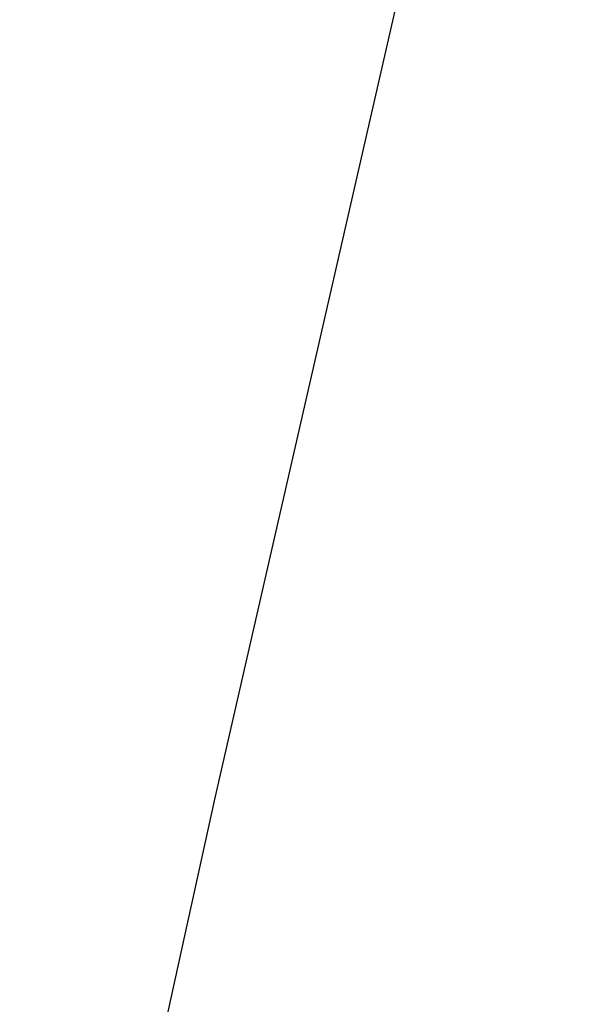
# Model space of a CAD drawing. Units: inches. Extents: x 3590 to 5167, y 65 to 1917.
# Tile 87 of 100: x 5052.2777 to 5052.5773, y 1788.0928 to 1788.6144. Entities that reach past the tile are written whole.
import ezdxf

# ---------------------------------------------------------------- set-up
doc = ezdxf.new("R2010")
doc.units = ezdxf.units.IN
for name, color, linetype, lineweight in [('A-ANNO-DIMS', 2, 'Continuous', 18), ('A-FLOR-PATT', 8, 'Continuous', 13), ('L-PLNT', 94, 'Continuous', 18)]:
    doc.layers.add(name, color=color, linetype=linetype, lineweight=lineweight)
doc.layers.add('DIENHOA', color=3, linetype='Continuous')
doc.styles.get("Standard").update_dxf_attribs({"font": 'arial.ttf'})
doc.dimstyles.new('ISO-25', dxfattribs={"dimtxt": 9, "dimasz": 2.5, "dimexe": 1.25, "dimexo": 0.625, "dimtad": 1, "dimdec": 1, "dimlunit": 3, "dimtxsty": 'Standard', "dimcen": 2.5, "dimadec": 0, "dimazin": 0, "dimtfac": 1, "dimtdec": 1, "dimtmove": 0, "dimatfit": 3, "dimfxl": 1, "dimarcsym": 0})

# ---------------------------------------------------------------- blocks, each defined once
blk = doc.blocks.new('Cay03_mb')
at = {"layer": 'DIENHOA'}
blk.add_lwpolyline([(112.868, 491.948), (95.994, 419.691), (79.461, 347.371), (63.915, 276.46), (50.006, 208.43), (38.381, 144.752), (29.688, 86.901), (24.574, 36.346), (23.687, -5.439)], dxfattribs=at)
blk = doc.blocks.new('*D322')
at = {"layer": 'A-ANNO-DIMS', "color": 0, "lineweight": -2, "transparency": 16777216}
for p, q in [((5035.74373, 1766.18424), (5035.74373, 1761.19899)), ((5064.81203, 1766.18424), (5064.81203, 1761.19899)), ((5038.24373, 1762.44899), (5062.31203, 1762.44899)), ((5064.81203, 1762.44899), (5166.99109, 1762.44899))]:
    blk.add_line(p, q, dxfattribs=at)
at = {"layer": 'A-ANNO-DIMS', "color": 0, "transparency": 16777216}
for points in [[(5038.24373, 1762.86566), (5038.24373, 1762.03233), (5035.74373, 1762.44899)], [(5062.31203, 1762.86566), (5062.31203, 1762.03233), (5064.81203, 1762.44899)]]:
    blk.add_solid(points, dxfattribs=at)
at = {"layer": 'Defpoints', "color": 0, "transparency": 16777216}
for p in [(5035.74373, 1766.80924), (5064.81203, 1766.80924), (5064.81203, 1762.44899)]:
    blk.add_point(p, dxfattribs=at)
at = {"layer": 'A-ANNO-DIMS', "color": 0, "transparency": 16777216, "insert": (5117.15156, 1767.66915), "char_height": 9, "attachment_point": 5}
blk.add_mtext('PLANT 2\'-5" TYP.', dxfattribs=at)

msp = doc.modelspace()

# ---------------------------------------------------------------- hatches: boundary and pattern name
at = {"layer": 'A-FLOR-PATT', "transparency": 33554687}
h = msp.add_hatch(dxfattribs=at)
h.set_pattern_fill('AR-HBONE', color=256, scale=0.2)
h.set_pattern_definition([(45, (-588.972, 0), (0, 28.73682), [60.96, -20.32]), (135, (-574.604, 14.368), (3e-15, 28.73682), [60.96, -20.32])])
h.paths.add_polyline_path([(5071.27403, 1796.99898), (4933.27403, 1796.99898), (4933.27403, 1753.99898), (4962.77403, 1753.99898, -0.414214), (4928.77403, 1719.99898), (4933.27403, 1718.99898), (4933.27403, 1334.99898), (5071.27403, 1334.99898)])
h.paths.add_polyline_path([(4951.78002, 1521.0767), (4951.7151, 1521.0404), (4951.56345, 1520.89532)], flags=16)
h.paths.add_polyline_path([(4952.267, 1521.37645), (4952.1977, 1521.37111), (4952.19823, 1521.35558)], flags=0)
h.paths.add_polyline_path([(4967.05076, 1529.72832), (4965.23122, 1528.69444), (4963.41109, 1527.71401), (4961.75649, 1526.85081), (4963.58887, 1527.44938), (4964.03555, 1527.47802), (4962.9755, 1527.24902), (4961.76022, 1526.85203), (4959.79219, 1525.83406), (4958.00498, 1524.89483), (4956.24031, 1523.92961), (4954.50395, 1522.91854), (4954.1294, 1522.68163), (4953.36051, 1521.99688), (4953.36558, 1521.99754), (4953.605, 1522.06367), (4955.10605, 1522.76083), (4956.92108, 1523.43405), (4958.67784, 1523.91513), (4960.35834, 1524.20036), (4961.94456, 1524.28606), (4964.17144, 1524.10849), (4965.95752, 1523.30903), (4963.86273, 1522.97565), (4965.18742, 1522.49898), (4963.36614, 1522.49715), (4961.54526, 1522.48682), (4959.76359, 1522.46077), (4958.30414, 1522.4188), (4957.97356, 1522.38829), (4956.30692, 1522.2324), (4954.71821, 1522.07143), (4953.25077, 1521.89915), (4953.52509, 1521.62277), (4954.33087, 1521.37883), (4956.24263, 1521.22987), (4958.03913, 1520.92952), (4959.68424, 1520.48339), (4961.16007, 1519.89569), (4963.10699, 1518.80022), (4964.39286, 1517.32518), (4962.97306, 1517.72596), (4964.55841, 1516.66059), (4965.40664, 1515.70779), (4963.50733, 1516.32179), (4961.67995, 1517.0051), (4959.93478, 1517.74489), (4958.2821, 1518.52833), (4956.73216, 1519.34257), (4955.29527, 1520.17478), (4954.67155, 1520.57237), (4954.51279, 1520.6271), (4955.65848, 1519.31837), (4956.70263, 1517.98232), (4957.64403, 1516.64663), (4958.48545, 1515.33439), (4959.54998, 1513.52398), (4960.43768, 1511.76936), (4958.84107, 1513.6196), (4957.45175, 1515.3249), (4955.8186, 1517.45855), (4956.66537, 1515.44764), (4957.11109, 1513.92292), (4957.44681, 1511.71434), (4957.07641, 1509.79288), (4956.53757, 1511.1103), (4955.99231, 1512.56892), (4955.44448, 1514.12509), (4954.89794, 1515.73518), (4954.35653, 1517.35553), (4953.82412, 1518.94251), (4953.30455, 1520.45247), (4953.06452, 1521.11563), (4952.97143, 1521.14607), (4952.94932, 1521.08646), (4952.72981, 1520.19905), (4953.3698, 1518.02364), (4953.75708, 1516.37279), (4954.05124, 1514.76538), (4954.26449, 1513.22121), (4954.47124, 1511.13121), (4954.4971, 1510.40174), (4954.40903, 1511.76006), (4954.26449, 1513.22121), (4954.05124, 1514.76538), (4953.75708, 1516.37279), (4953.3698, 1518.02364), (4952.87718, 1519.69813), (4952.7161, 1520.1412), (4952.53301, 1519.05871), (4952.37428, 1517.78881), (4952.21925, 1516.31167), (4952.04598, 1514.59986), (4951.83253, 1512.62598), (4951.55697, 1510.36259), (4951.20331, 1512.16818), (4950.85168, 1514.33931), (4950.98529, 1516.37594), (4951.6596, 1518.28625), (4952.59261, 1520.48085), (4952.35664, 1521.1299), (4951.85502, 1520.32753), (4950.83901, 1518.90828), (4949.77675, 1517.58658), (4948.91554, 1516.61731), (4948.11099, 1515.2561), (4947.0891, 1513.55389), (4945.88937, 1511.61495), (4946.32587, 1513.40232), (4946.5624, 1514.24913), (4945.52771, 1513.32668), (4944.58105, 1512.53126), (4946.01774, 1514.50825), (4947.2044, 1516.04763), (4947.89331, 1517.31331), (4949.30686, 1518.76446), (4950.41417, 1519.76716), (4950.45131, 1519.80628), (4952.267, 1521.37645), (4951.64457, 1521.49317), (4950.40371, 1521.17954), (4948.04447, 1520.35868), (4946.11863, 1519.45198), (4944.57182, 1518.47484), (4943.34962, 1517.44265), (4941.99695, 1515.91971), (4941.66146, 1515.27475), (4942.81332, 1516.98973), (4944.57182, 1518.47484), (4946.11863, 1519.45198), (4948.04447, 1520.35868), (4950.40371, 1521.17954), (4951.64457, 1521.49317), (4949.64678, 1521.86781), (4948.59979, 1521.75633), (4947.12629, 1521.5699), (4945.42015, 1521.34763), (4943.44969, 1521.10462), (4941.18319, 1520.85596), (4942.86028, 1521.61265), (4943.87308, 1522.03014), (4942.95216, 1521.9093), (4941.40968, 1521.48512), (4939.54287, 1520.67019), (4938.96775, 1520.2255), (4940.73284, 1521.29899), (4942.95216, 1521.9093), (4943.70184, 1522.00767), (4945.89419, 1522.69998), (4947.56488, 1522.71399), (4948.92086, 1522.56573), (4951.13144, 1522.18271), (4950.97062, 1522.2969), (4948.12924, 1523.00563), (4946.03496, 1523.70671), (4944.23235, 1524.52143), (4942.70692, 1525.46111), (4941.44419, 1526.53707), (4940.42968, 1527.76062), (4939.6489, 1529.14306), (4941.42091, 1528.12232), (4943.14742, 1527.13248), (4944.84093, 1526.17457), (4946.51394, 1525.24959), (4948.17893, 1524.35855), (4948.36457, 1524.26336), (4946.47531, 1526.04459), (4945.18083, 1527.54042), (4944.19039, 1529.03339), (4943.49559, 1530.53985), (4943.27808, 1531.3597), (4942.49849, 1531.91903), (4943.11353, 1531.76249), (4942.95927, 1533.6586), (4944.13953, 1531.9886), (4944.61171, 1531.32339), (4946.20163, 1530.46341), (4947.48567, 1529.50925), (4948.79027, 1528.22649), (4950.36754, 1526.23746), (4949.48547, 1528.15549), (4948.85128, 1530.12254), (4948.49054, 1532.04127), (4948.38105, 1533.91822), (4948.50062, 1535.7599), (4948.82704, 1537.57284), (4949.41803, 1535.56526), (4949.95684, 1533.56932), (4950.46414, 1531.5861), (4950.96058, 1529.6167), (4951.3911, 1527.95448), (4951.72352, 1530.68689), (4952.20106, 1532.57994), (4952.88914, 1534.32964), (4953.77035, 1535.95123), (4954.82726, 1537.45995), (4954.52145, 1535.38966), (4954.27314, 1533.93684), (4955.57999, 1535.6627), (4956.74758, 1536.73859), (4956.15852, 1534.78029), (4955.58917, 1532.87334), (4955.04336, 1531.00581), (4954.52493, 1529.16576), (4954.03771, 1527.34127), (4953.63833, 1525.73298), (4953.61143, 1525.58564), (4953.39805, 1524.16565), (4953.38219, 1524.00887), (4954.06955, 1525.47563), (4954.91212, 1527.02173), (4956.13627, 1528.89351), (4957.84668, 1530.57701), (4959.37601, 1531.54014), (4958.25596, 1530.10398), (4957.14284, 1528.66291), (4956.06626, 1527.24305), (4955.05579, 1525.87054), (4954.14104, 1524.57149), (4953.35159, 1523.37204), (4953.31079, 1523.30299), (4953.27253, 1522.92478), (4953.26102, 1522.38213), (4954.1031, 1523.37273), (4954.63005, 1524.28376), (4955.96149, 1526.35767), (4957.23002, 1528.12969), (4958.42057, 1529.60864), (4960.03671, 1531.36792), (4961.3736, 1532.3752), (4962.1015, 1532.77), (4961.06994, 1531.06113), (4959.98733, 1529.43811), (4958.86851, 1527.90803), (4958.15046, 1527.00742), (4959.80291, 1528.00314), (4961.58854, 1528.79257), (4963.39087, 1529.32783), (4965.21118, 1529.63205)], flags=16)
h.paths.add_polyline_path([(4962.94387, 1523.18187), (4961.10714, 1523.42192), (4960.39205, 1523.36158), (4962.34964, 1523.33061)], flags=0)
h.paths.add_polyline_path([(5049.54129, 1584.55089), (5049.47636, 1584.51458), (5049.32471, 1584.3695)], flags=16)
h.paths.add_polyline_path([(5050.02827, 1584.85063), (5049.95897, 1584.84529), (5049.95949, 1584.82976)], flags=0)
h.paths.add_polyline_path([(5042.33308, 1581.94902), (5043.8799, 1582.92616), (5045.80573, 1583.83286), (5048.16498, 1584.65372), (5049.40583, 1584.96736), (5047.40804, 1585.34199), (5046.36106, 1585.23052), (5044.88755, 1585.04408), (5043.18142, 1584.82181), (5041.21095, 1584.5788), (5038.94446, 1584.33014), (5040.62155, 1585.08683), (5041.63434, 1585.50432), (5040.71343, 1585.38348), (5039.17095, 1584.9593), (5037.30414, 1584.14438), (5036.72901, 1583.69969), (5038.4941, 1584.77317), (5040.71343, 1585.38348), (5041.4631, 1585.48185), (5043.65545, 1586.17416), (5045.32615, 1586.18818), (5046.68212, 1586.03992), (5048.8927, 1585.6569), (5048.73188, 1585.77108), (5045.89051, 1586.47981), (5043.79622, 1587.18089), (5041.99361, 1587.99561), (5040.46818, 1588.9353), (5039.20546, 1590.01125), (5038.19095, 1591.2348), (5037.41016, 1592.61725), (5039.18217, 1591.5965), (5040.90868, 1590.60667), (5042.6022, 1589.64876), (5044.2752, 1588.72378), (5045.94019, 1587.83274), (5046.12584, 1587.73754), (5044.23658, 1589.51878), (5042.9421, 1591.01461), (5041.95166, 1592.50757), (5041.25685, 1594.01403), (5041.03935, 1594.83388), (5040.25976, 1595.39321), (5040.8748, 1595.23667), (5040.72054, 1597.13279), (5041.9008, 1595.46278), (5042.37297, 1594.79758), (5043.96289, 1593.93759), (5045.24694, 1592.98344), (5046.55153, 1591.70068), (5048.12881, 1589.71164), (5047.24673, 1591.62967), (5046.61254, 1593.59672), (5046.2518, 1595.51546), (5046.14232, 1597.3924), (5046.26189, 1599.23408), (5046.5883, 1601.04703), (5047.17929, 1599.03944), (5047.71811, 1597.0435), (5048.22541, 1595.06028), (5048.72184, 1593.09089), (5049.15237, 1591.42866), (5049.48478, 1594.16107), (5049.96233, 1596.05412), (5050.65041, 1597.80382), (5051.53161, 1599.42541), (5052.58852, 1600.93414), (5052.28271, 1598.86384), (5052.03441, 1597.41102), (5053.34126, 1599.13689), (5054.50884, 1600.21277), (5053.91979, 1598.25447), (5053.35044, 1596.34752), (5052.80463, 1594.47999), (5052.2862, 1592.63995), (5051.79898, 1590.81546), (5051.39959, 1589.20716), (5051.3727, 1589.05983), (5051.15931, 1587.63984), (5051.14346, 1587.48305), (5051.83082, 1588.94982), (5052.67339, 1590.49592), (5053.89754, 1592.3677), (5055.60794, 1594.05119), (5057.13728, 1595.01432), (5056.01722, 1593.57817), (5054.90411, 1592.1371), (5053.82752, 1590.71724), (5052.81705, 1589.34472), (5051.9023, 1588.04567), (5051.11286, 1586.84622), (5051.07205, 1586.77718), (5051.03379, 1586.39896), (5051.02228, 1585.85631), (5051.86437, 1586.84692), (5052.39131, 1587.75794), (5053.72275, 1589.83185), (5054.99128, 1591.60387), (5056.18183, 1593.08282), (5057.79798, 1594.84211), (5059.13486, 1595.84938), (5059.86276, 1596.24419), (5058.83121, 1594.53531), (5057.7486, 1592.9123), (5056.62978, 1591.38221), (5055.91173, 1590.4816), (5057.56418, 1591.47732), (5059.34981, 1592.26675), (5061.15214, 1592.80202), (5062.97245, 1593.10624), (5064.81203, 1593.20251), (5062.99248, 1592.16863), (5061.17235, 1591.18819), (5059.51775, 1590.325), (5061.35014, 1590.92356), (5061.79682, 1590.95221), (5060.73676, 1590.7232), (5059.52148, 1590.32622), (5057.55345, 1589.30825), (5055.76625, 1588.36901), (5054.00157, 1587.40379), (5052.26521, 1586.39273), (5051.89067, 1586.15581), (5051.12177, 1585.47106), (5051.12684, 1585.47172), (5051.36627, 1585.53786), (5052.86732, 1586.23502), (5054.68234, 1586.90824), (5056.4391, 1587.38931), (5058.1196, 1587.67454), (5059.70582, 1587.76024), (5061.93271, 1587.58268), (5063.71878, 1586.78321), (5061.62399, 1586.44983), (5062.94869, 1585.97317), (5061.12741, 1585.97133), (5059.30653, 1585.961), (5057.52486, 1585.93496), (5056.06541, 1585.89299), (5055.73482, 1585.86247), (5054.06819, 1585.70658), (5052.47947, 1585.54561), (5051.01204, 1585.37333), (5051.28635, 1585.09695), (5052.09214, 1584.85301), (5054.00389, 1584.70406), (5055.8004, 1584.4037), (5057.44551, 1583.95757), (5058.92133, 1583.36987), (5060.86825, 1582.27441), (5062.15413, 1580.79937), (5060.73433, 1581.20015), (5062.31967, 1580.13477), (5063.1679, 1579.18198), (5061.2686, 1579.79597), (5059.44122, 1580.47928), (5057.69605, 1581.21908), (5056.04336, 1582.00251), (5054.49343, 1582.81675), (5053.05653, 1583.64897), (5052.43281, 1584.04656), (5052.27405, 1584.10128), (5053.41974, 1582.79255), (5054.4639, 1581.4565), (5055.40529, 1580.12081), (5056.24672, 1578.80858), (5057.31125, 1576.99816), (5058.19895, 1575.24354), (5056.60234, 1577.09378), (5055.21301, 1578.79908), (5053.57987, 1580.93274), (5054.42664, 1578.92183), (5054.87235, 1577.3971), (5055.20808, 1575.18852), (5054.83767, 1573.26706), (5054.29883, 1574.58448), (5053.75357, 1576.0431), (5053.20575, 1577.59927), (5052.6592, 1579.20936), (5052.1178, 1580.82971), (5051.58538, 1582.41669), (5051.06582, 1583.92666), (5050.82578, 1584.58981), (5050.7327, 1584.62025), (5050.71058, 1584.56064), (5050.49108, 1583.67323), (5051.13107, 1581.49782), (5051.51835, 1579.84698), (5051.8125, 1578.23957), (5052.02575, 1576.69539), (5052.23251, 1574.6054), (5052.25836, 1573.87593), (5052.1703, 1575.23424), (5052.02575, 1576.69539), (5051.8125, 1578.23957), (5051.51835, 1579.84698), (5051.13107, 1581.49782), (5050.63844, 1583.17231), (5050.47736, 1583.61538), (5050.29428, 1582.53289), (5050.13554, 1581.26299), (5049.98051, 1579.78585), (5049.80724, 1578.07405), (5049.59379, 1576.10016), (5049.31823, 1573.83678), (5048.96458, 1575.64237), (5048.61294, 1577.8135), (5048.74656, 1579.85012), (5049.42086, 1581.76043), (5050.35388, 1583.95503), (5050.1179, 1584.60408), (5049.61629, 1583.80172), (5048.60027, 1582.38246), (5047.53801, 1581.06076), (5046.67681, 1580.09149), (5045.87225, 1578.73029), (5044.85036, 1577.02808), (5043.65063, 1575.08913), (5044.08713, 1576.8765), (5044.32366, 1577.72331), (5043.28898, 1576.80086), (5042.34232, 1576.00545), (5043.779, 1577.98243), (5044.96566, 1579.52182), (5045.65457, 1580.78749), (5047.06813, 1582.23865), (5048.17543, 1583.24134), (5048.21258, 1583.28047), (5050.02827, 1584.85063), (5049.40583, 1584.96736), (5048.16498, 1584.65372), (5045.80573, 1583.83286), (5043.8799, 1582.92616), (5042.33308, 1581.94902), (5041.11088, 1580.91684), (5039.75821, 1579.39389), (5039.42272, 1578.74894), (5040.57458, 1580.46391)], flags=16)
h.paths.add_polyline_path([(4954.79872, 1533.12029), (4954.26249, 1532.07935), (4953.83112, 1530.93464), (4953.50472, 1529.63602), (4953.28338, 1528.13331), (4953.16721, 1526.37637), (4953.15631, 1524.31504), (4953.27669, 1521.23629), (4952.80168, 1521.84177), (4951.55695, 1521.99789), (4950.97575, 1521.9613), (4952.66059, 1521.94097), (4952.80168, 1521.84177), (4953.15249, 1523.59258), (4953.16721, 1526.37637), (4953.28338, 1528.13331), (4953.60929, 1530.34598), (4954.45558, 1532.59174)], flags=0)
h.paths.add_polyline_path([(5050.56294, 1585.31596), (5049.31822, 1585.47208), (5048.73702, 1585.43548), (5050.42186, 1585.41516), (5050.56294, 1585.31596), (5050.91375, 1587.06676), (5050.92848, 1589.85056), (5051.04465, 1591.6075), (5051.37055, 1593.82017), (5052.21684, 1596.06593), (5052.55999, 1596.59447), (5052.02375, 1595.55353), (5051.59238, 1594.40883), (5051.26598, 1593.1102), (5051.04465, 1591.6075), (5050.92848, 1589.85056), (5050.91757, 1587.78922), (5051.03795, 1584.71048)], flags=0)
h.paths.add_polyline_path([(5058.15332, 1586.83576), (5060.11091, 1586.80479), (5060.70514, 1586.65605), (5058.8684, 1586.8961)], flags=0)
h.paths.add_polyline_path([(5049.54129, 1430.93611), (5049.47636, 1430.8998), (5049.32471, 1430.75472)], flags=16)
h.paths.add_polyline_path([(5050.02827, 1431.23585), (5049.95897, 1431.23051), (5049.95949, 1431.21498)], flags=0)
h.paths.add_polyline_path([(5046.5883, 1447.43225), (5047.17929, 1445.42467), (5047.71811, 1443.42872), (5048.22541, 1441.4455), (5048.72184, 1439.47611), (5049.15237, 1437.81388), (5049.48478, 1440.5463), (5049.96233, 1442.43934), (5050.65041, 1444.18904), (5051.53161, 1445.81063), (5052.58852, 1447.31936), (5052.28271, 1445.24906), (5052.03441, 1443.79624), (5053.34126, 1445.52211), (5054.50884, 1446.59799), (5053.91979, 1444.63969), (5053.35044, 1442.73274), (5052.80463, 1440.86521), (5052.2862, 1439.02517), (5051.79898, 1437.20068), (5051.39959, 1435.59238), (5051.3727, 1435.44505), (5051.15931, 1434.02506), (5051.14346, 1433.86828), (5051.83082, 1435.33504), (5052.67339, 1436.88114), (5053.89754, 1438.75292), (5055.60794, 1440.43641), (5057.13728, 1441.39954), (5056.01722, 1439.96339), (5054.90411, 1438.52232), (5053.82752, 1437.10246), (5052.81705, 1435.72994), (5051.9023, 1434.4309), (5051.11286, 1433.23145), (5051.07205, 1433.1624), (5051.03379, 1432.78418), (5051.02228, 1432.24153), (5051.86437, 1433.23214), (5052.39131, 1434.14316), (5053.72275, 1436.21707), (5054.99128, 1437.98909), (5056.18183, 1439.46805), (5057.79798, 1441.22733), (5059.13486, 1442.23461), (5059.86276, 1442.62941), (5058.83121, 1440.92053), (5057.7486, 1439.29752), (5056.62978, 1437.76743), (5055.91173, 1436.86682), (5057.56418, 1437.86255), (5059.34981, 1438.65197), (5061.15214, 1439.18724), (5062.97245, 1439.49146), (5064.81203, 1439.58773), (5062.99248, 1438.55385), (5061.17235, 1437.57342), (5059.51775, 1436.71022), (5061.35014, 1437.30879), (5061.79682, 1437.33743), (5060.73676, 1437.10842), (5059.52148, 1436.71144), (5057.55345, 1435.69347), (5055.76625, 1434.75423), (5054.00157, 1433.78901), (5052.26521, 1432.77795), (5051.89067, 1432.54103), (5051.12177, 1431.85628), (5051.12684, 1431.85694), (5051.36627, 1431.92308), (5052.86732, 1432.62024), (5054.68234, 1433.29346), (5056.4391, 1433.77453), (5058.1196, 1434.05976), (5059.70582, 1434.14546), (5061.93271, 1433.9679), (5063.71878, 1433.16843), (5061.62399, 1432.83505), (5062.94869, 1432.35839), (5061.12741, 1432.35655), (5059.30653, 1432.34623), (5057.52486, 1432.32018), (5056.06541, 1432.27821), (5055.73482, 1432.24769), (5054.06819, 1432.09181), (5052.47947, 1431.93083), (5051.01204, 1431.75856), (5051.28635, 1431.48218), (5052.09214, 1431.23823), (5054.00389, 1431.08928), (5055.8004, 1430.78892), (5057.44551, 1430.34279), (5058.92133, 1429.75509), (5060.86825, 1428.65963), (5062.15413, 1427.18459), (5060.73433, 1427.58537), (5062.31967, 1426.52), (5063.1679, 1425.5672), (5061.2686, 1426.18119), (5059.44122, 1426.86451), (5057.69605, 1427.6043), (5056.04336, 1428.38773), (5054.49343, 1429.20197), (5053.05653, 1430.03419), (5052.43281, 1430.43178), (5052.27405, 1430.48651), (5053.41974, 1429.17777), (5054.4639, 1427.84172), (5055.40529, 1426.50603), (5056.24672, 1425.1938), (5057.31125, 1423.38338), (5058.19895, 1421.62877), (5056.60234, 1423.479), (5055.21301, 1425.1843), (5053.57987, 1427.31796), (5054.42664, 1425.30705), (5054.87235, 1423.78233), (5055.20808, 1421.57374), (5054.83767, 1419.65228), (5054.29883, 1420.9697), (5053.75357, 1422.42832), (5053.20575, 1423.9845), (5052.6592, 1425.59458), (5052.1178, 1427.21493), (5051.58538, 1428.80191), (5051.06582, 1430.31188), (5050.82578, 1430.97503), (5050.7327, 1431.00547), (5050.71058, 1430.94586), (5050.49108, 1430.05845), (5051.13107, 1427.88305), (5051.51835, 1426.2322), (5051.8125, 1424.62479), (5052.02575, 1423.08061), (5052.23251, 1420.99062), (5052.25836, 1420.26115), (5052.1703, 1421.61947), (5052.02575, 1423.08061), (5051.8125, 1424.62479), (5051.51835, 1426.2322), (5051.13107, 1427.88305), (5050.63844, 1429.55753), (5050.47736, 1430.0006), (5050.29428, 1428.91811), (5050.13554, 1427.64821), (5049.98051, 1426.17107), (5049.80724, 1424.45927), (5049.59379, 1422.48539), (5049.31823, 1420.222), (5048.96458, 1422.02759), (5048.61294, 1424.19872), (5048.74656, 1426.23534), (5049.42086, 1428.14565), (5050.35388, 1430.34025), (5050.1179, 1430.98931), (5049.61629, 1430.18694), (5048.60027, 1428.76768), (5047.53801, 1427.44598), (5046.67681, 1426.47671), (5045.87225, 1425.11551), (5044.85036, 1423.4133), (5043.65063, 1421.47435), (5044.08713, 1423.26172), (5044.32366, 1424.10854), (5043.28898, 1423.18608), (5042.34232, 1422.39067), (5043.779, 1424.36765), (5044.96566, 1425.90704), (5045.65457, 1427.17272), (5047.06813, 1428.62387), (5048.17543, 1429.62657), (5048.21258, 1429.66569), (5050.02827, 1431.23585), (5049.40583, 1431.35258), (5048.16498, 1431.03894), (5045.80573, 1430.21809), (5043.8799, 1429.31139), (5042.33308, 1428.33424), (5041.11088, 1427.30206), (5039.75821, 1425.77911), (5039.42272, 1425.13416), (5040.57458, 1426.84914), (5042.33308, 1428.33424), (5043.8799, 1429.31139), (5045.80573, 1430.21809), (5048.16498, 1431.03894), (5049.40583, 1431.35258), (5047.40804, 1431.72722), (5046.36106, 1431.61574), (5044.88755, 1431.42931), (5043.18142, 1431.20704), (5041.21095, 1430.96402), (5038.94446, 1430.71536), (5040.62155, 1431.47205), (5041.63434, 1431.88954), (5040.71343, 1431.76871), (5039.17095, 1431.34453), (5037.30414, 1430.5296), (5036.72901, 1430.08491), (5038.4941, 1431.1584), (5040.71343, 1431.76871), (5041.4631, 1431.86707), (5043.65545, 1432.55939), (5045.32615, 1432.5734), (5046.68212, 1432.42514), (5048.8927, 1432.04212), (5048.73188, 1432.1563), (5045.89051, 1432.86503), (5043.79622, 1433.56611), (5041.99361, 1434.38083), (5040.46818, 1435.32052), (5039.20546, 1436.39648), (5038.19095, 1437.62002), (5037.41016, 1439.00247), (5039.18217, 1437.98172), (5040.90868, 1436.99189), (5042.6022, 1436.03398), (5044.2752, 1435.109), (5045.94019, 1434.21796), (5046.12584, 1434.12276), (5044.23658, 1435.904), (5042.9421, 1437.39983), (5041.95166, 1438.8928), (5041.25685, 1440.39925), (5041.03935, 1441.2191), (5040.25976, 1441.77844), (5040.8748, 1441.62189), (5040.72054, 1443.51801), (5041.9008, 1441.848), (5042.37297, 1441.1828), (5043.96289, 1440.32282), (5045.24694, 1439.36866), (5046.55153, 1438.0859), (5048.12881, 1436.09686), (5047.24673, 1438.01489), (5046.61254, 1439.98195), (5046.2518, 1441.90068), (5046.14232, 1443.77762), (5046.26189, 1445.6193)], flags=16)
h.paths.add_polyline_path([(5052.38176, 1444.25496), (5051.62263, 1442.77987), (5052.02375, 1441.93875), (5052.55999, 1442.9797)], flags=0)
h.paths.add_polyline_path([(5050.56294, 1431.70118), (5049.31822, 1431.8573), (5048.73702, 1431.82071), (5050.42186, 1431.80038)], flags=0)
h.paths.add_polyline_path([(5058.15332, 1433.22098), (5060.11091, 1433.19001), (5060.70514, 1433.04127), (5058.8684, 1433.28132)], flags=0)
h.paths.add_polyline_path([(5049.54129, 1352.28535), (5049.47636, 1352.24904), (5049.32471, 1352.10396)], flags=16)
h.paths.add_polyline_path([(5050.02827, 1352.58509), (5049.95897, 1352.57975), (5049.95949, 1352.56422)], flags=0)
h.paths.add_polyline_path([(5046.5883, 1368.78149), (5047.17929, 1366.7739), (5047.71811, 1364.77796), (5048.22541, 1362.79474), (5048.72184, 1360.82534), (5049.15237, 1359.16312), (5049.48478, 1361.89553), (5049.96233, 1363.78858), (5050.65041, 1365.53828), (5051.53161, 1367.15987), (5052.58852, 1368.6686), (5052.28271, 1366.5983), (5052.03441, 1365.14548), (5053.34126, 1366.87135), (5054.50884, 1367.94723), (5053.91979, 1365.98893), (5053.35044, 1364.08198), (5052.80463, 1362.21445), (5052.2862, 1360.37441), (5051.79898, 1358.54992), (5051.39959, 1356.94162), (5051.3727, 1356.79428), (5051.15931, 1355.37429), (5051.14346, 1355.21751), (5051.83082, 1356.68428), (5052.67339, 1358.23037), (5053.89754, 1360.10216), (5055.60794, 1361.78565), (5057.13728, 1362.74878), (5056.01722, 1361.31262), (5054.90411, 1359.87155), (5053.82752, 1358.4517), (5052.81705, 1357.07918), (5051.9023, 1355.78013), (5051.11286, 1354.58068), (5051.07205, 1354.51164), (5051.03379, 1354.13342), (5051.02228, 1353.59077), (5051.86437, 1354.58137), (5052.39131, 1355.4924), (5053.72275, 1357.56631), (5054.99128, 1359.33833), (5056.18183, 1360.81728), (5057.79798, 1362.57656), (5059.13486, 1363.58384), (5059.86276, 1363.97864), (5058.83121, 1362.26977), (5057.7486, 1360.64675), (5056.62978, 1359.11667), (5055.91173, 1358.21606), (5057.56418, 1359.21178), (5059.34981, 1360.00121), (5061.15214, 1360.53648), (5062.97245, 1360.84069), (5064.81203, 1360.93697), (5062.99248, 1359.90308), (5061.17235, 1358.92265), (5059.51775, 1358.05946), (5061.35014, 1358.65802), (5061.79682, 1358.68666), (5060.73676, 1358.45766), (5059.52148, 1358.06068), (5057.55345, 1357.0427), (5055.76625, 1356.10347), (5054.00157, 1355.13825), (5052.26521, 1354.12718), (5051.89067, 1353.89027), (5051.12177, 1353.20552), (5051.12684, 1353.20618), (5051.36627, 1353.27231), (5052.86732, 1353.96947), (5054.68234, 1354.6427), (5056.4391, 1355.12377), (5058.1196, 1355.409), (5059.70582, 1355.4947), (5061.93271, 1355.31713), (5063.71878, 1354.51767), (5061.62399, 1354.18429), (5062.94869, 1353.70763), (5061.12741, 1353.70579), (5059.30653, 1353.69546), (5057.52486, 1353.66942), (5056.06541, 1353.62744), (5055.73482, 1353.59693), (5054.06819, 1353.44104), (5052.47947, 1353.28007), (5051.01204, 1353.10779), (5051.28635, 1352.83141), (5052.09214, 1352.58747), (5054.00389, 1352.43852), (5055.8004, 1352.13816), (5057.44551, 1351.69203), (5058.92133, 1351.10433), (5060.86825, 1350.00887), (5062.15413, 1348.53382), (5060.73433, 1348.9346), (5062.31967, 1347.86923), (5063.1679, 1346.91643), (5061.2686, 1347.53043), (5059.44122, 1348.21374), (5057.69605, 1348.95353), (5056.04336, 1349.73697), (5054.49343, 1350.55121), (5053.05653, 1351.38342), (5052.43281, 1351.78101), (5052.27405, 1351.83574), (5053.41974, 1350.52701), (5054.4639, 1349.19096), (5055.40529, 1347.85527), (5056.24672, 1346.54303), (5057.31125, 1344.73262), (5058.19895, 1342.978), (5056.60234, 1344.82824), (5055.21301, 1346.53354), (5053.57987, 1348.6672), (5054.42664, 1346.65629), (5054.87235, 1345.13156), (5055.20808, 1342.92298), (5054.83767, 1341.00152), (5054.29883, 1342.31894), (5053.75357, 1343.77756), (5053.20575, 1345.33373), (5052.6592, 1346.94382), (5052.1178, 1348.56417), (5051.58538, 1350.15115), (5051.06582, 1351.66111), (5050.82578, 1352.32427), (5050.7327, 1352.35471), (5050.71058, 1352.2951), (5050.49108, 1351.40769), (5051.13107, 1349.23228), (5051.51835, 1347.58144), (5051.8125, 1345.97403), (5052.02575, 1344.42985), (5052.23251, 1342.33986), (5052.25836, 1341.61039), (5052.1703, 1342.9687), (5052.02575, 1344.42985), (5051.8125, 1345.97403), (5051.51835, 1347.58144), (5051.13107, 1349.23228), (5050.63844, 1350.90677), (5050.47736, 1351.34984), (5050.29428, 1350.26735), (5050.13554, 1348.99745), (5049.98051, 1347.52031), (5049.80724, 1345.80851), (5049.59379, 1343.83462), (5049.31823, 1341.57124), (5048.96458, 1343.37683), (5048.61294, 1345.54796), (5048.74656, 1347.58458), (5049.42086, 1349.49489), (5050.35388, 1351.68949), (5050.1179, 1352.33854), (5049.61629, 1351.53617), (5048.60027, 1350.11692), (5047.53801, 1348.79522), (5046.67681, 1347.82595), (5045.87225, 1346.46475), (5044.85036, 1344.76253), (5043.65063, 1342.82359), (5044.08713, 1344.61096), (5044.32366, 1345.45777), (5043.28898, 1344.53532), (5042.34232, 1343.7399), (5043.779, 1345.71689), (5044.96566, 1347.25627), (5045.65457, 1348.52195), (5047.06813, 1349.9731), (5048.17543, 1350.9758), (5048.21258, 1351.01493), (5050.02827, 1352.58509), (5049.40583, 1352.70181), (5048.16498, 1352.38818), (5045.80573, 1351.56732), (5043.8799, 1350.66062), (5042.33308, 1349.68348), (5041.11088, 1348.65129), (5039.75821, 1347.12835), (5039.42272, 1346.4834), (5040.57458, 1348.19837), (5042.33308, 1349.68348), (5043.8799, 1350.66062), (5045.80573, 1351.56732), (5048.16498, 1352.38818), (5049.40583, 1352.70181), (5047.40804, 1353.07645), (5046.36106, 1352.96498), (5044.88755, 1352.77854), (5043.18142, 1352.55627), (5041.21095, 1352.31326), (5038.94446, 1352.0646), (5040.62155, 1352.82129), (5041.63434, 1353.23878), (5040.71343, 1353.11794), (5039.17095, 1352.69376), (5037.30414, 1351.87884), (5036.72901, 1351.43415), (5038.4941, 1352.50763), (5040.71343, 1353.11794), (5041.4631, 1353.21631), (5043.65545, 1353.90862), (5045.32615, 1353.92263), (5046.68212, 1353.77438), (5048.8927, 1353.39136), (5048.73188, 1353.50554), (5045.89051, 1354.21427), (5043.79622, 1354.91535), (5041.99361, 1355.73007), (5040.46818, 1356.66975), (5039.20546, 1357.74571), (5038.19095, 1358.96926), (5037.41016, 1360.35171), (5039.18217, 1359.33096), (5040.90868, 1358.34112), (5042.6022, 1357.38321), (5044.2752, 1356.45824), (5045.94019, 1355.5672), (5046.12584, 1355.472), (5044.23658, 1357.25323), (5042.9421, 1358.74906), (5041.95166, 1360.24203), (5041.25685, 1361.74849), (5041.03935, 1362.56834), (5040.25976, 1363.12767), (5040.8748, 1362.97113), (5040.72054, 1364.86725), (5041.9008, 1363.19724), (5042.37297, 1362.53203), (5043.96289, 1361.67205), (5045.24694, 1360.7179), (5046.55153, 1359.43513), (5048.12881, 1357.4461), (5047.24673, 1359.36413), (5046.61254, 1361.33118), (5046.2518, 1363.24992), (5046.14232, 1365.12686), (5046.26189, 1366.96854)], flags=16)
h.paths.add_polyline_path([(5052.38176, 1365.6042), (5051.62263, 1364.12911), (5052.02375, 1363.28799), (5052.55999, 1364.32893)], flags=0)
h.paths.add_polyline_path([(4951.78002, 1698.04081), (4951.7151, 1698.0045), (4951.56345, 1697.85942)], flags=16)
h.paths.add_polyline_path([(4952.267, 1698.34055), (4952.1977, 1698.33521), (4952.19823, 1698.31968)], flags=0)
h.paths.add_polyline_path([(4957.07641, 1686.75698), (4956.53757, 1688.0744), (4955.99231, 1689.53302), (4955.44448, 1691.08919), (4954.89794, 1692.69928), (4954.35653, 1694.31963), (4953.82412, 1695.90661), (4953.30455, 1697.41658), (4953.06452, 1698.07973), (4952.97143, 1698.11017), (4952.94932, 1698.05056), (4952.72981, 1697.16315), (4953.3698, 1694.98774), (4953.75708, 1693.3369), (4954.05124, 1691.72949), (4954.26449, 1690.18531), (4954.47124, 1688.09532), (4954.4971, 1687.36585), (4954.40903, 1688.72416), (4954.26449, 1690.18531), (4954.05124, 1691.72949), (4953.75708, 1693.3369), (4953.3698, 1694.98774), (4952.87718, 1696.66223), (4952.7161, 1697.1053), (4952.53301, 1696.02281), (4952.37428, 1694.75291), (4952.21925, 1693.27577), (4952.04598, 1691.56397), (4951.83253, 1689.59008), (4951.55697, 1687.3267), (4951.20331, 1689.13229), (4950.85168, 1691.30342), (4950.98529, 1693.34004), (4951.6596, 1695.25035), (4952.59261, 1697.44495), (4952.35664, 1698.09401), (4951.85502, 1697.29164), (4950.83901, 1695.87238), (4949.77675, 1694.55068), (4948.91554, 1693.58141), (4948.11099, 1692.22021), (4947.0891, 1690.518), (4945.88937, 1688.57905), (4946.32587, 1690.36642), (4946.5624, 1691.21323), (4945.52771, 1690.29078), (4944.58105, 1689.49537), (4946.01774, 1691.47235), (4947.2044, 1693.01174), (4947.89331, 1694.27741), (4949.30686, 1695.72857), (4950.41417, 1696.73127), (4950.45131, 1696.77039), (4952.267, 1698.34055), (4951.64457, 1698.45728), (4950.40371, 1698.14364), (4948.04447, 1697.32278), (4946.11863, 1696.41608), (4944.57182, 1695.43894), (4943.34962, 1694.40676), (4941.99695, 1692.88381), (4941.66146, 1692.23886), (4942.81332, 1693.95383), (4944.57182, 1695.43894), (4946.11863, 1696.41608), (4948.04447, 1697.32278), (4950.40371, 1698.14364), (4951.64457, 1698.45728), (4949.64678, 1698.83191), (4948.59979, 1698.72044), (4947.12629, 1698.53401), (4945.42015, 1698.31174), (4943.44969, 1698.06872), (4941.18319, 1697.82006), (4942.86028, 1698.57675), (4943.87308, 1698.99424), (4942.95216, 1698.8734), (4941.40968, 1698.44922), (4939.54287, 1697.6343), (4938.96775, 1697.18961), (4940.73284, 1698.26309), (4942.95216, 1698.8734), (4943.70184, 1698.97177), (4945.89419, 1699.66409), (4947.56488, 1699.6781), (4948.92086, 1699.52984), (4951.13144, 1699.14682), (4950.97062, 1699.261), (4948.12924, 1699.96973), (4946.03496, 1700.67081), (4944.23235, 1701.48553), (4942.70692, 1702.42522), (4941.44419, 1703.50117), (4940.42968, 1704.72472), (4939.6489, 1706.10717), (4941.42091, 1705.08642), (4943.14742, 1704.09659), (4944.84093, 1703.13868), (4946.51394, 1702.2137), (4948.17893, 1701.32266), (4948.36457, 1701.22746), (4946.47531, 1703.0087), (4945.18083, 1704.50453), (4944.19039, 1705.9975), (4943.49559, 1707.50395), (4943.27808, 1708.3238), (4942.49849, 1708.88314), (4943.11353, 1708.72659), (4942.95927, 1710.62271), (4944.13953, 1708.9527), (4944.61171, 1708.2875), (4946.20163, 1707.42751), (4947.48567, 1706.47336), (4948.79027, 1705.1906), (4950.36754, 1703.20156), (4949.48547, 1705.11959), (4948.85128, 1707.08664), (4948.49054, 1709.00538), (4948.38105, 1710.88232), (4948.50062, 1712.724), (4948.82704, 1714.53695), (4949.41803, 1712.52937), (4949.95684, 1710.53342), (4950.46414, 1708.5502), (4950.96058, 1706.58081), (4951.3911, 1704.91858), (4951.72352, 1707.65099), (4952.20106, 1709.54404), (4952.88914, 1711.29374), (4953.77035, 1712.91533), (4954.82726, 1714.42406), (4954.52145, 1712.35376), (4954.27314, 1710.90094), (4955.57999, 1712.62681), (4956.74758, 1713.70269), (4956.15852, 1711.74439), (4955.58917, 1709.83744), (4955.04336, 1707.96991), (4954.52493, 1706.12987), (4954.03771, 1704.30538), (4953.63833, 1702.69708), (4953.61143, 1702.54975), (4953.39805, 1701.12976), (4953.38219, 1700.97297), (4954.06955, 1702.43974), (4954.91212, 1703.98584), (4956.13627, 1705.85762), (4957.84668, 1707.54111), (4959.37601, 1708.50424), (4958.25596, 1707.06809), (4957.14284, 1705.62702), (4956.06626, 1704.20716), (4955.05579, 1702.83464), (4954.14104, 1701.53559), (4953.35159, 1700.33614), (4953.31079, 1700.2671), (4953.27253, 1699.88888), (4953.26102, 1699.34623), (4954.1031, 1700.33684), (4954.63005, 1701.24786), (4955.96149, 1703.32177), (4957.23002, 1705.09379), (4958.42057, 1706.57274), (4960.03671, 1708.33203), (4961.3736, 1709.33931), (4962.1015, 1709.73411), (4961.06994, 1708.02523), (4959.98733, 1706.40222), (4958.86851, 1704.87213), (4958.15046, 1703.97152), (4959.80291, 1704.96725), (4961.58854, 1705.75667), (4963.39087, 1706.29194), (4965.21118, 1706.59616), (4967.05076, 1706.69243), (4965.23122, 1705.65855), (4963.41109, 1704.67811), (4961.75649, 1703.81492), (4963.58887, 1704.41349), (4964.03555, 1704.44213), (4962.9755, 1704.21312), (4961.76022, 1703.81614), (4959.79219, 1702.79817), (4958.00498, 1701.85893), (4956.24031, 1700.89371), (4954.50395, 1699.88265), (4954.1294, 1699.64573), (4953.36051, 1698.96098), (4953.36558, 1698.96164), (4953.605, 1699.02778), (4955.10605, 1699.72494), (4956.92108, 1700.39816), (4958.67784, 1700.87923), (4960.35834, 1701.16446), (4961.94456, 1701.25016), (4964.17144, 1701.0726), (4965.95752, 1700.27313), (4963.86273, 1699.93975), (4965.18742, 1699.46309), (4963.36614, 1699.46125), (4961.54526, 1699.45092), (4959.76359, 1699.42488), (4958.30414, 1699.38291), (4957.97356, 1699.35239), (4956.30692, 1699.1965), (4954.71821, 1699.03553), (4953.25077, 1698.86326), (4953.52509, 1698.58688), (4954.33087, 1698.34293), (4956.24263, 1698.19398), (4958.03913, 1697.89362), (4959.68424, 1697.44749), (4961.16007, 1696.85979), (4963.10699, 1695.76433), (4964.39286, 1694.28929), (4962.97306, 1694.69007), (4964.55841, 1693.6247), (4965.40664, 1692.6719), (4963.50733, 1693.28589), (4961.67995, 1693.9692), (4959.93478, 1694.709), (4958.2821, 1695.49243), (4956.73216, 1696.30667), (4955.29527, 1697.13889), (4954.67155, 1697.53648), (4954.51279, 1697.5912), (4955.65848, 1696.28247), (4956.70263, 1694.94642), (4957.64403, 1693.61073), (4958.48545, 1692.2985), (4959.54998, 1690.48808), (4960.43768, 1688.73346), (4958.84107, 1690.5837), (4957.45175, 1692.289), (4955.8186, 1694.42266), (4956.66537, 1692.41175), (4957.11109, 1690.88702), (4957.44681, 1688.67844)], flags=16)
h.paths.add_polyline_path([(5050.56294, 1353.05042), (5049.31822, 1353.20654), (5048.73702, 1353.16994), (5050.42186, 1353.14961)], flags=0)
h.paths.add_polyline_path([(4951.78002, 1351.48609), (4951.7151, 1351.44979), (4951.56345, 1351.30471)], flags=16)
h.paths.add_polyline_path([(4952.267, 1351.78584), (4952.1977, 1351.7805), (4952.19823, 1351.76497)], flags=0)
h.paths.add_polyline_path([(4954.82726, 1367.86934), (4954.52145, 1365.79905), (4954.27314, 1364.34623), (4955.57999, 1366.07209), (4956.74758, 1367.14798), (4956.15852, 1365.18968), (4955.58917, 1363.28273), (4955.04336, 1361.4152), (4954.52493, 1359.57515), (4954.03771, 1357.75066), (4953.63833, 1356.14237), (4953.61143, 1355.99503), (4953.39805, 1354.57504), (4953.38219, 1354.41826), (4954.06955, 1355.88503), (4954.91212, 1357.43112), (4956.13627, 1359.3029), (4957.84668, 1360.9864), (4959.37601, 1361.94953), (4958.25596, 1360.51337), (4957.14284, 1359.0723), (4956.06626, 1357.65245), (4955.05579, 1356.27993), (4954.14104, 1354.98088), (4953.35159, 1353.78143), (4953.31079, 1353.71238), (4953.27253, 1353.33417), (4953.26102, 1352.79152), (4954.1031, 1353.78212), (4954.63005, 1354.69315), (4955.96149, 1356.76706), (4957.23002, 1358.53908), (4958.42057, 1360.01803), (4960.03671, 1361.77731), (4961.3736, 1362.78459), (4962.1015, 1363.17939), (4961.06994, 1361.47052), (4959.98733, 1359.8475), (4958.86851, 1358.31742), (4958.15046, 1357.41681), (4959.80291, 1358.41253), (4961.58854, 1359.20196), (4963.39087, 1359.73723), (4965.21118, 1360.04144), (4967.05076, 1360.13771), (4965.23122, 1359.10383), (4963.41109, 1358.1234), (4961.75649, 1357.26021), (4963.58887, 1357.85877), (4964.03555, 1357.88741), (4962.9755, 1357.65841), (4961.76022, 1357.26143), (4959.79219, 1356.24345), (4958.00498, 1355.30422), (4956.24031, 1354.339), (4954.50395, 1353.32793), (4954.1294, 1353.09102), (4953.36051, 1352.40627), (4953.36558, 1352.40693), (4953.605, 1352.47306), (4955.10605, 1353.17022), (4956.92108, 1353.84345), (4958.67784, 1354.32452), (4960.35834, 1354.60975), (4961.94456, 1354.69545), (4964.17144, 1354.51788), (4965.95752, 1353.71842), (4963.86273, 1353.38504), (4965.18742, 1352.90838), (4963.36614, 1352.90654), (4961.54526, 1352.89621), (4959.76359, 1352.87016), (4958.30414, 1352.82819), (4957.97356, 1352.79768), (4956.30692, 1352.64179), (4954.71821, 1352.48082), (4953.25077, 1352.30854), (4953.52509, 1352.03216), (4954.33087, 1351.78822), (4956.24263, 1351.63926), (4958.03913, 1351.33891), (4959.68424, 1350.89278), (4961.16007, 1350.30508), (4963.10699, 1349.20961), (4964.39286, 1347.73457), (4962.97306, 1348.13535), (4964.55841, 1347.06998), (4965.40664, 1346.11718), (4963.50733, 1346.73118), (4961.67995, 1347.41449), (4959.93478, 1348.15428), (4958.2821, 1348.93772), (4956.73216, 1349.75196), (4955.29527, 1350.58417), (4954.67155, 1350.98176), (4954.51279, 1351.03649), (4955.65848, 1349.72776), (4956.70263, 1348.39171), (4957.64403, 1347.05602), (4958.48545, 1345.74378), (4959.54998, 1343.93337), (4960.43768, 1342.17875), (4958.84107, 1344.02899), (4957.45175, 1345.73429), (4955.8186, 1347.86795), (4956.66537, 1345.85703), (4957.11109, 1344.33231), (4957.44681, 1342.12373), (4957.07641, 1340.20227), (4956.53757, 1341.51969), (4955.99231, 1342.97831), (4955.44448, 1344.53448), (4954.89794, 1346.14457), (4954.35653, 1347.76492), (4953.82412, 1349.3519), (4953.30455, 1350.86186), (4953.06452, 1351.52502), (4952.97143, 1351.55546), (4952.94932, 1351.49585), (4952.72981, 1350.60844), (4953.3698, 1348.43303), (4953.75708, 1346.78218), (4954.05124, 1345.17477), (4954.26449, 1343.6306), (4954.47124, 1341.5406), (4954.4971, 1340.81113), (4954.40903, 1342.16945), (4954.26449, 1343.6306), (4954.05124, 1345.17477), (4953.75708, 1346.78218), (4953.3698, 1348.43303), (4952.87718, 1350.10752), (4952.7161, 1350.55059), (4952.53301, 1349.4681), (4952.37428, 1348.1982), (4952.21925, 1346.72106), (4952.04598, 1345.00926), (4951.83253, 1343.03537), (4951.55697, 1340.77198), (4951.20331, 1342.57757), (4950.85168, 1344.7487), (4950.98529, 1346.78533), (4951.6596, 1348.69564), (4952.59261, 1350.89024), (4952.35664, 1351.53929), (4951.85502, 1350.73692), (4950.83901, 1349.31767), (4949.77675, 1347.99597), (4948.91554, 1347.0267), (4948.11099, 1345.66549), (4947.0891, 1343.96328), (4945.88937, 1342.02434), (4946.32587, 1343.81171), (4946.5624, 1344.65852), (4945.52771, 1343.73607), (4944.58105, 1342.94065), (4946.01774, 1344.91764), (4947.2044, 1346.45702), (4947.89331, 1347.7227), (4949.30686, 1349.17385), (4950.41417, 1350.17655), (4950.45131, 1350.21567), (4952.267, 1351.78584), (4951.64457, 1351.90256), (4950.40371, 1351.58893), (4948.04447, 1350.76807), (4946.11863, 1349.86137), (4944.57182, 1348.88423), (4943.34962, 1347.85204), (4941.99695, 1346.3291), (4941.66146, 1345.68414), (4942.81332, 1347.39912), (4944.57182, 1348.88423), (4946.11863, 1349.86137), (4948.04447, 1350.76807), (4950.40371, 1351.58893), (4951.64457, 1351.90256), (4949.64678, 1352.2772), (4948.59979, 1352.16572), (4947.12629, 1351.97929), (4945.42015, 1351.75702), (4943.44969, 1351.51401), (4941.18319, 1351.26535), (4942.86028, 1352.02204), (4943.87308, 1352.43953), (4942.95216, 1352.31869), (4941.40968, 1351.89451), (4939.54287, 1351.07958), (4938.96775, 1350.63489), (4940.73284, 1351.70838), (4942.95216, 1352.31869), (4943.70184, 1352.41706), (4945.89419, 1353.10937), (4947.56488, 1353.12338), (4948.92086, 1352.97513), (4951.13144, 1352.59211), (4950.97062, 1352.70629), (4948.12924, 1353.41502), (4946.03496, 1354.1161), (4944.23235, 1354.93082), (4942.70692, 1355.8705), (4941.44419, 1356.94646), (4940.42968, 1358.17001), (4939.6489, 1359.55246), (4941.42091, 1358.53171), (4943.14742, 1357.54187), (4944.84093, 1356.58396), (4946.51394, 1355.65898), (4948.17893, 1354.76794), (4948.36457, 1354.67275), (4946.47531, 1356.45398), (4945.18083, 1357.94981), (4944.19039, 1359.44278), (4943.49559, 1360.94924), (4943.27808, 1361.76909), (4942.49849, 1362.32842), (4943.11353, 1362.17188), (4942.95927, 1364.06799), (4944.13953, 1362.39799), (4944.61171, 1361.73278), (4946.20163, 1360.8728), (4947.48567, 1359.91864), (4948.79027, 1358.63588), (4950.36754, 1356.64685), (4949.48547, 1358.56488), (4948.85128, 1360.53193), (4948.49054, 1362.45066), (4948.38105, 1364.32761), (4948.50062, 1366.16929), (4948.82704, 1367.98223), (4949.41803, 1365.97465), (4949.95684, 1363.97871), (4950.46414, 1361.99549), (4950.96058, 1360.02609), (4951.3911, 1358.36387), (4951.72352, 1361.09628), (4952.20106, 1362.98933), (4952.88914, 1364.73903), (4953.77035, 1366.36062)], flags=16)
h.paths.add_polyline_path([(4954.79872, 1363.52968), (4954.26249, 1362.48874), (4953.83112, 1361.34403), (4953.50472, 1360.04541), (4953.28338, 1358.54271), (4953.16721, 1356.78577), (4953.15631, 1354.72443), (4953.27669, 1351.64568), (4952.80168, 1352.25116), (4951.55695, 1352.40728), (4950.97575, 1352.37069), (4952.66059, 1352.35036), (4952.80168, 1352.25116), (4953.15249, 1354.00197), (4953.16721, 1356.78577), (4953.28338, 1358.54271), (4953.60929, 1360.75537), (4954.45558, 1363.00113)], flags=0)
h.paths.add_polyline_path([(4952.80168, 1698.80588), (4951.55695, 1698.962), (4950.97575, 1698.92541), (4952.66059, 1698.90508), (4952.80168, 1698.80588), (4953.15249, 1700.55668), (4953.16721, 1703.34048), (4953.28338, 1705.09742), (4953.60929, 1707.31009), (4954.45558, 1709.55585), (4954.79872, 1710.0844), (4954.26249, 1709.04345), (4953.83112, 1707.89875), (4953.50472, 1706.60012), (4953.28338, 1705.09742), (4953.16721, 1703.34048), (4953.15631, 1701.27914), (4953.27669, 1698.2004)], flags=0)
h.paths.add_polyline_path([(4962.94387, 1700.14597), (4961.10714, 1700.38602), (4960.39205, 1700.32568), (4962.34964, 1700.29471)], flags=0)
h.paths.add_polyline_path([(5058.15332, 1354.57022), (5060.11091, 1354.53925), (5060.70514, 1354.39051), (5058.8684, 1354.63056)], flags=0)
h.paths.add_polyline_path([(4962.94387, 1353.59126), (4961.10714, 1353.83131), (4960.39205, 1353.77097), (4962.34964, 1353.74)], flags=0)
h.paths.add_polyline_path([(5049.54129, 1778.71989), (5049.47636, 1778.68358), (5049.32471, 1778.5385)], flags=16)
h.paths.add_polyline_path([(5050.02827, 1779.01963), (5049.95897, 1779.01429), (5049.95949, 1778.99876)], flags=0)
h.paths.add_polyline_path([(5052.25836, 1768.04493), (5052.1703, 1769.40324), (5052.02575, 1770.86439), (5051.8125, 1772.40857), (5051.51835, 1774.01598), (5051.13107, 1775.66682), (5050.63844, 1777.34131), (5050.47736, 1777.78438), (5050.29428, 1776.70189), (5050.13554, 1775.43199), (5049.98051, 1773.95485), (5049.80724, 1772.24305), (5049.59379, 1770.26916), (5049.31823, 1768.00578), (5048.96458, 1769.81137), (5048.61294, 1771.9825), (5048.74656, 1774.01912), (5049.42086, 1775.92943), (5050.35388, 1778.12403), (5050.1179, 1778.77309), (5049.61629, 1777.97072), (5048.60027, 1776.55146), (5047.53801, 1775.22976), (5046.67681, 1774.26049), (5045.87225, 1772.89929), (5044.85036, 1771.19708), (5043.65063, 1769.25813), (5044.08713, 1771.0455), (5044.32366, 1771.89231), (5043.28898, 1770.96986), (5042.34232, 1770.17445), (5043.779, 1772.15143), (5044.96566, 1773.69082), (5045.65457, 1774.95649), (5047.06813, 1776.40765), (5048.17543, 1777.41035), (5048.21258, 1777.44947), (5050.02827, 1779.01963), (5049.40583, 1779.13636), (5048.16498, 1778.82272), (5045.80573, 1778.00187), (5043.8799, 1777.09516), (5042.33308, 1776.11802), (5041.11088, 1775.08584), (5039.75821, 1773.56289), (5039.42272, 1772.91794), (5040.57458, 1774.63291), (5042.33308, 1776.11802), (5043.8799, 1777.09516), (5045.80573, 1778.00187), (5048.16498, 1778.82272), (5049.40583, 1779.13636), (5047.40804, 1779.51099), (5046.36106, 1779.39952), (5044.88755, 1779.21309), (5043.18142, 1778.99082), (5041.21095, 1778.7478), (5038.94446, 1778.49914), (5040.62155, 1779.25583), (5041.63434, 1779.67332), (5040.71343, 1779.55248), (5039.17095, 1779.1283), (5037.30414, 1778.31338), (5036.72901, 1777.86869), (5038.4941, 1778.94217), (5040.71343, 1779.55248), (5041.4631, 1779.65085), (5043.65545, 1780.34317), (5045.32615, 1780.35718), (5046.68212, 1780.20892), (5048.8927, 1779.8259), (5048.73188, 1779.94008), (5045.89051, 1780.64881), (5043.79622, 1781.34989), (5041.99361, 1782.16461), (5040.46818, 1783.1043), (5039.20546, 1784.18025), (5038.19095, 1785.4038), (5037.41016, 1786.78625), (5039.18217, 1785.7655), (5040.90868, 1784.77567), (5042.6022, 1783.81776), (5044.2752, 1782.89278), (5045.94019, 1782.00174), (5046.12584, 1781.90654), (5044.23658, 1783.68778), (5042.9421, 1785.18361), (5041.95166, 1786.67658), (5041.25685, 1788.18303), (5041.03935, 1789.00288), (5040.25976, 1789.56222), (5040.8748, 1789.40567), (5040.72054, 1791.30179), (5041.9008, 1789.63178), (5042.37297, 1788.96658), (5043.96289, 1788.10659), (5045.24694, 1787.15244), (5046.55153, 1785.86968), (5048.12881, 1783.88064), (5047.24673, 1785.79867), (5046.61254, 1787.76572), (5046.2518, 1789.68446), (5046.14232, 1791.5614), (5046.26189, 1793.40308), (5046.5883, 1795.21603), (5047.17929, 1793.20845), (5047.71811, 1791.2125), (5048.22541, 1789.22928), (5048.72184, 1787.25989), (5049.15237, 1785.59766), (5049.48478, 1788.33007), (5049.96233, 1790.22312), (5050.65041, 1791.97282), (5051.53161, 1793.59441), (5052.58852, 1795.10314), (5052.28271, 1793.03284), (5052.03441, 1791.58002), (5053.34126, 1793.30589), (5054.50884, 1794.38177), (5053.91979, 1792.42347), (5053.35044, 1790.51652), (5052.80463, 1788.64899), (5052.2862, 1786.80895), (5051.79898, 1784.98446), (5051.39959, 1783.37616), (5051.3727, 1783.22883), (5051.15931, 1781.80884), (5051.14346, 1781.65205), (5051.83082, 1783.11882), (5052.67339, 1784.66492), (5053.89754, 1786.5367), (5055.60794, 1788.22019), (5057.13728, 1789.18332), (5056.01722, 1787.74717), (5054.90411, 1786.3061), (5053.82752, 1784.88624), (5052.81705, 1783.51372), (5051.9023, 1782.21467), (5051.11286, 1781.01522), (5051.07205, 1780.94618), (5051.03379, 1780.56796), (5051.02228, 1780.02531), (5051.86437, 1781.01592), (5052.39131, 1781.92694), (5053.72275, 1784.00085), (5054.99128, 1785.77287), (5056.18183, 1787.25182), (5057.79798, 1789.01111), (5059.13486, 1790.01839), (5059.86276, 1790.41319), (5058.83121, 1788.70431), (5057.7486, 1787.0813), (5056.62978, 1785.55121), (5055.91173, 1784.6506), (5057.56418, 1785.64633), (5059.34981, 1786.43575), (5061.15214, 1786.97102), (5062.97245, 1787.27524), (5064.81203, 1787.37151), (5062.99248, 1786.33763), (5061.17235, 1785.35719), (5059.51775, 1784.494), (5061.35014, 1785.09257), (5061.79682, 1785.12121), (5060.73676, 1784.8922), (5059.52148, 1784.49522), (5057.55345, 1783.47725), (5055.76625, 1782.53801), (5054.00157, 1781.57279), (5052.26521, 1780.56173), (5051.89067, 1780.32481), (5051.12177, 1779.64006), (5051.12684, 1779.64072), (5051.36627, 1779.70686), (5052.86732, 1780.40402), (5054.68234, 1781.07724), (5056.4391, 1781.55831), (5058.1196, 1781.84354), (5059.70582, 1781.92924), (5061.93271, 1781.75168), (5063.71878, 1780.95221), (5061.62399, 1780.61883), (5062.94869, 1780.14217), (5061.12741, 1780.14033), (5059.30653, 1780.13), (5057.52486, 1780.10396), (5056.06541, 1780.06199), (5055.73482, 1780.03147), (5054.06819, 1779.87558), (5052.47947, 1779.71461), (5051.01204, 1779.54234), (5051.28635, 1779.26596), (5052.09214, 1779.02201), (5054.00389, 1778.87306), (5055.8004, 1778.5727), (5057.44551, 1778.12657), (5058.92133, 1777.53887), (5060.86825, 1776.44341), (5062.15413, 1774.96837), (5060.73433, 1775.36915), (5062.31967, 1774.30378), (5063.1679, 1773.35098), (5061.2686, 1773.96497), (5059.44122, 1774.64828), (5057.69605, 1775.38808), (5056.04336, 1776.17151), (5054.49343, 1776.98575), (5053.05653, 1777.81797), (5052.43281, 1778.21556), (5052.27405, 1778.27028), (5053.41974, 1776.96155), (5054.4639, 1775.6255), (5055.40529, 1774.28981), (5056.24672, 1772.97758), (5057.31125, 1771.16716), (5058.19895, 1769.41254), (5056.60234, 1771.26278), (5055.21301, 1772.96808), (5053.57987, 1775.10174), (5054.42664, 1773.09083), (5054.87235, 1771.5661), (5055.20808, 1769.35752), (5054.83767, 1767.43606), (5054.29883, 1768.75348), (5053.75357, 1770.2121), (5053.20575, 1771.76827), (5052.6592, 1773.37836), (5052.1178, 1774.99871), (5051.58538, 1776.58569), (5051.06582, 1778.09566), (5050.82578, 1778.75881), (5050.7327, 1778.78925), (5050.71058, 1778.72964), (5050.49108, 1777.84223), (5051.13107, 1775.66682), (5051.51835, 1774.01598), (5051.8125, 1772.40857), (5052.02575, 1770.86439), (5052.23251, 1768.7744)], flags=16)
h.paths.add_polyline_path([(5050.56294, 1779.48496), (5049.31822, 1779.64108), (5048.73702, 1779.60449), (5050.42186, 1779.58416), (5050.56294, 1779.48496), (5050.91375, 1781.23576), (5050.92848, 1784.01956), (5051.04465, 1785.7765), (5051.37055, 1787.98917), (5052.21684, 1790.23493), (5052.55999, 1790.76348), (5052.02375, 1789.72253), (5051.59238, 1788.57783), (5051.26598, 1787.2792), (5051.04465, 1785.7765), (5050.92848, 1784.01956), (5050.91757, 1781.95822), (5051.03795, 1778.87948)], flags=0)
h.paths.add_polyline_path([(5058.15332, 1781.00476), (5060.11091, 1780.97379), (5060.70514, 1780.82505), (5058.8684, 1781.0651)], flags=0)

# ---------------------------------------------------------------- block references
at = {"layer": 'L-PLNT', "xscale": 0.0245452446402784, "yscale": 0.0245452446402784, "zscale": 0.0245452446402784}
msp.add_blockref('Cay03_mb', (5050.43062, 1779.67584), dxfattribs=at)

# ---------------------------------------------------------------- dimensions: what is measured, and where the dimension line sits
at = {"layer": 'A-ANNO-DIMS'}
dim = msp.add_linear_dim(base=(5064.81203, 1762.44899), p1=(5035.74373, 1766.80924), p2=(5064.81203, 1766.80924), text='PLANT <> TYP.', dimstyle='ISO-25', override={"dimdec": 1, "dimlfac": 1, "dimrnd": 0, "dimzin": 1, "dimdsep": 46, "dimlunit": 4, "dimfrac": 2}, dxfattribs=at)
dim.commit()
dim.dimension.update_dxf_attribs({"geometry": '*D322', "text_midpoint": (5117.15156, 1767.66915)})

doc.saveas('drawing.dxf')
